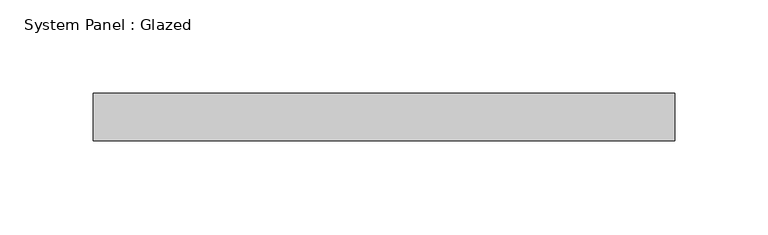
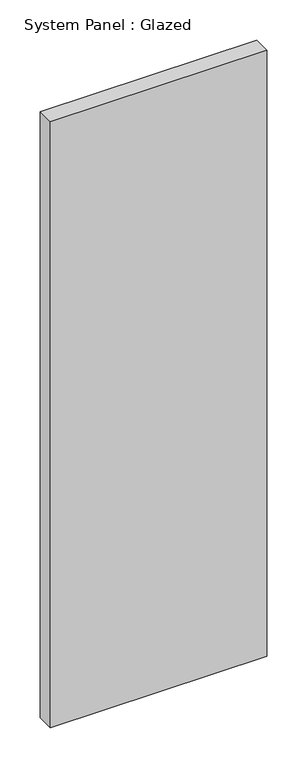
"""IFC4 building model written with IfcOpenShell, lengths in millimetres: plate geometry, System Panel : Glazed."""

from ifc_helpers import new_model, si_unit, origin, origin_with_axes, place, context, project, spatial, polyline, outline, extrude, source, transform, mapped, element, save


def system_panel_glazed_60bba13d(model_context):
    return source(origin(), model_context, "Body", "SweptSolid", [
        extrude(outline(polyline([(155.575, 19.05), (-155.575, 19.05), (-155.575, 44.45), (155.575, 44.45), (155.575, 19.05)])), origin_with_axes(), (0.0, 0.0, 1.0), 920.75),
    ])


if __name__ == "__main__":
    model = new_model("IFC4")
    model_context = context("Model", 3, world=origin())
    ifc_project = project(units=[si_unit("LENGTHUNIT", "METRE", prefix="MILLI")], contexts=[model_context])
    site = spatial("IfcSite", under=ifc_project)
    building = spatial("IfcBuilding", under=site)
    placement = place(None, origin())
    system_panel_glazed_shape = system_panel_glazed_60bba13d(model_context)
    element("IfcPlate", 1, ObjectType="System Panel : Glazed", at=placement, inside=building, context=model_context, shape_type="MappedRepresentation", body=[
        mapped(system_panel_glazed_shape, transform((0.0, 0.0, 0.0), x_axis=(1.0, 0.0, 0.0), y_axis=(0.0, 1.0, 0.0), z_axis=(0.0, 0.0, 1.0))),
    ])
    save(model, "model.ifc")

# Revit data of these elements
# Type "System Panel : Glazed"
#   Construction Type Id = "GSP4R"
#   Analytic Construction = "1/8 in Pilkington single glazing"
#   Visual Light Transmittance = 0.9
#   Solar Heat Gain Coefficient = 0.86
#   Heat Transfer Coefficient (U) = 1.18115 BTU/(h·ft²·°F)
#   Define Thermal Properties by = 1
# Element 1 (IfcPlate, "System Panel : Glazed")
#   Materials on its faces: "Glass"
# Materials
#   "Glass": class "Glass", colour RGB 0 128 192, transparency 0.75, Description = "Soda Lime Glass", Cost = 0
